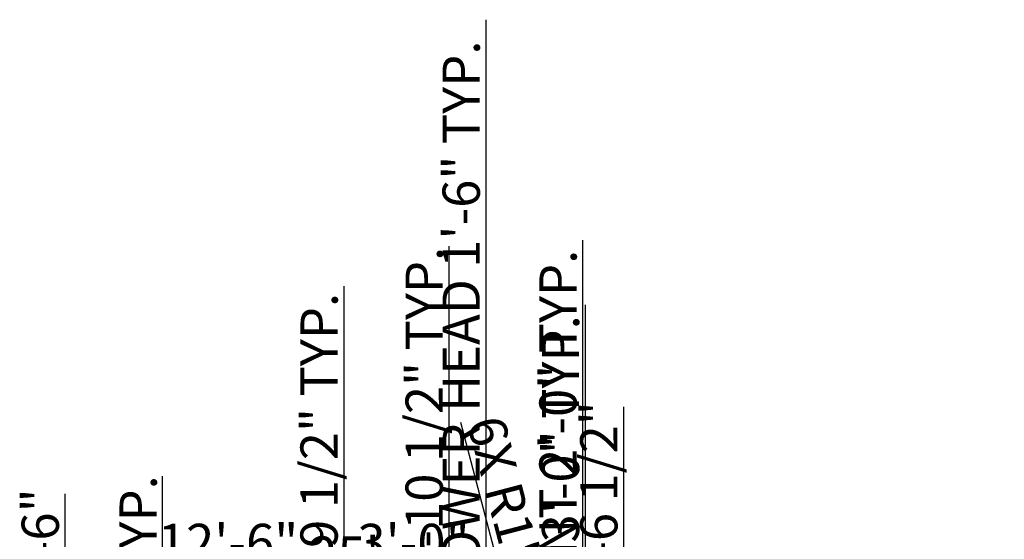
# Model space of a CAD drawing. Units: inches. Extents: x 830 to 1639, y 2591 to 3595.
# Tile 7 of 7: x 922 to 1557, y 3260 to 3595. Entities that reach past the tile are written whole.
import ezdxf

# ---------------------------------------------------------------- set-up
doc = ezdxf.new("R2010")
doc.units = ezdxf.units.IN
doc.layers.add('A-ANNO-DIMS', color=2, linetype='Continuous', lineweight=18)
doc.styles.get("Standard").update_dxf_attribs({"font": 'arial.ttf'})
doc.dimstyles.new('ISO-25', dxfattribs={"dimtxt": 24, "dimasz": 12, "dimexe": 1.25, "dimexo": 0.625, "dimtad": 1, "dimdec": 0, "dimlunit": 3, "dimtxsty": 'Standard', "dimcen": 2.5, "dimadec": 0, "dimazin": 0, "dimtfac": 1, "dimtdec": 0, "dimtmove": 0, "dimatfit": 3, "dimfxl": 1, "dimarcsym": 0})

# ---------------------------------------------------------------- blocks, each defined once
blk = doc.blocks.new('*D15')
at = {"layer": 'A-ANNO-DIMS', "color": 0, "lineweight": -2, "transparency": 16777216}
for p, q in [((981.59, 3212.71), (981.59, 3235.25)), ((993.59, 3234), (1269.59, 3234)), ((1281.59, 3212.71), (1281.59, 3235.25))]:
    blk.add_line(p, q, dxfattribs=at)
at = {"layer": 'A-ANNO-DIMS', "color": 0, "transparency": 16777216}
for points in [[(993.59, 3236), (993.59, 3232), (981.59, 3234)], [(1269.59, 3236), (1269.59, 3232), (1281.59, 3234)]]:
    blk.add_solid(points, dxfattribs=at)
at = {"layer": 'Defpoints', "color": 0, "transparency": 16777216}
for p in [(1281.59, 3234), (981.59, 3212.09), (1281.59, 3212.09)]:
    blk.add_point(p, dxfattribs=at)
at = {"layer": 'A-ANNO-DIMS', "color": 0, "transparency": 16777216, "insert": (1131.59, 3246.88), "char_height": 24, "attachment_point": 5}
blk.add_mtext("25'", dxfattribs=at)
blk = doc.blocks.new('*D22')
at = {"layer": 'A-ANNO-DIMS', "color": 0, "lineweight": -2, "transparency": 16777216}
for p, q in [((1286.99, 3094.42), (1286.99, 3411.37)), ((1282.21, 3094.42), (1288.24, 3094.42)), ((1286.99, 3070.42), (1286.99, 3082.42)), ((1282.21, 3058.42), (1288.24, 3058.42))]:
    blk.add_line(p, q, dxfattribs=at)
at = {"layer": 'A-ANNO-DIMS', "color": 0, "transparency": 16777216}
for points in [[(1284.99, 3082.42), (1288.99, 3082.42), (1286.99, 3094.42)], [(1284.99, 3070.42), (1288.99, 3070.42), (1286.99, 3058.42)]]:
    blk.add_solid(points, dxfattribs=at)
at = {"layer": 'Defpoints', "color": 0, "transparency": 16777216}
for p in [(1281.59, 3094.42), (1286.99, 3094.42), (1281.59, 3058.42)]:
    blk.add_point(p, dxfattribs=at)
at = {"layer": 'A-ANNO-DIMS', "color": 0, "transparency": 16777216, "insert": (1273.94, 3258.89), "char_height": 24, "attachment_point": 5, "rotation": 90}
blk.add_mtext('WINDOW 3\'-0" TYP.', dxfattribs=at)
blk = doc.blocks.new('*D24')
at = {"layer": 'A-ANNO-DIMS', "color": 0, "lineweight": -2, "transparency": 16777216}
for p, q in [((1285.19, 3193.45), (1285.19, 3452.97)), ((1282.21, 3181.45), (1286.44, 3181.45)), ((1285.19, 3157.45), (1285.19, 3181.45)), ((1282.21, 3157.45), (1286.44, 3157.45)), ((1285.19, 3145.45), (1285.19, 3133.45))]:
    blk.add_line(p, q, dxfattribs=at)
at = {"layer": 'A-ANNO-DIMS', "color": 0, "transparency": 16777216}
for points in [[(1283.19, 3193.45), (1287.19, 3193.45), (1285.19, 3181.45)], [(1283.19, 3145.45), (1287.19, 3145.45), (1285.19, 3157.45)]]:
    blk.add_solid(points, dxfattribs=at)
at = {"layer": 'Defpoints', "color": 0, "transparency": 16777216}
for p in [(1281.59, 3181.45), (1285.19, 3181.45), (1281.59, 3157.45)]:
    blk.add_point(p, dxfattribs=at)
at = {"layer": 'A-ANNO-DIMS', "color": 0, "transparency": 16777216, "insert": (1272.31, 3329.21), "char_height": 24, "attachment_point": 5, "rotation": 90}
blk.add_mtext('VENT 2\'-0" TYP.', dxfattribs=at)
blk = doc.blocks.new('*D27')
at = {"layer": 'A-ANNO-DIMS', "color": 0, "lineweight": -2, "transparency": 16777216}
for p, q in [((1014.41, 3143.5), (1014.41, 3300.79)), ((1011.93, 3131.5), (1015.66, 3131.5)), ((1014.41, 3112.26), (1014.41, 3131.5)), ((1011.93, 3112.26), (1015.66, 3112.26)), ((1014.41, 3100.26), (1014.41, 3088.26))]:
    blk.add_line(p, q, dxfattribs=at)
at = {"layer": 'A-ANNO-DIMS', "color": 0, "transparency": 16777216}
for points in [[(1012.41, 3143.5), (1016.41, 3143.5), (1014.41, 3131.5)], [(1012.41, 3100.26), (1016.41, 3100.26), (1014.41, 3112.26)]]:
    blk.add_solid(points, dxfattribs=at)
at = {"layer": 'Defpoints', "color": 0, "transparency": 16777216}
for p in [(1011.31, 3131.5), (1014.41, 3131.5), (1011.31, 3112.26)]:
    blk.add_point(p, dxfattribs=at)
at = {"layer": 'A-ANNO-DIMS', "color": 0, "transparency": 16777216, "insert": (1001.73, 3228.15), "char_height": 24, "attachment_point": 5, "rotation": 90}
blk.add_mtext('1\'-7" TYP.', dxfattribs=at)
blk = doc.blocks.new('*D34')
at = {"layer": 'A-ANNO-DIMS', "color": 0, "lineweight": -2, "transparency": 16777216}
for p, q in [((1189.9, 3205.85), (1177.9, 3205.85)), ((1201.9, 3203.69), (1201.9, 3207.1)), ((1201.9, 3205.85), (1220.46, 3205.85)), ((1220.46, 3203.69), (1220.46, 3207.1)), ((1232.46, 3205.85), (1556.8, 3205.85))]:
    blk.add_line(p, q, dxfattribs=at)
at = {"layer": 'A-ANNO-DIMS', "color": 0, "transparency": 16777216}
for points in [[(1189.9, 3207.85), (1189.9, 3203.85), (1201.9, 3205.85)], [(1232.46, 3207.85), (1232.46, 3203.85), (1220.46, 3205.85)]]:
    blk.add_solid(points, dxfattribs=at)
at = {"layer": 'Defpoints', "color": 0, "transparency": 16777216}
for p in [(1220.46, 3205.85), (1201.9, 3203.07), (1220.46, 3203.07)]:
    blk.add_point(p, dxfattribs=at)
at = {"layer": 'A-ANNO-DIMS', "color": 0, "transparency": 16777216, "insert": (1400.63, 3218.88), "char_height": 24, "attachment_point": 5}
blk.add_mtext('BASIN 1\'-6 1/2" TYP.', dxfattribs=at)
blk = doc.blocks.new('*D35')
at = {"layer": 'A-ANNO-DIMS', "color": 0, "lineweight": -2, "transparency": 16777216}
for p, q in [((1199.11, 3215.07), (1199.11, 3449.18)), ((1201.27, 3203.07), (1197.86, 3203.07)), ((1199.11, 3192.62), (1199.11, 3203.07)), ((1201.27, 3192.62), (1197.86, 3192.62)), ((1199.11, 3180.62), (1199.11, 3168.62))]:
    blk.add_line(p, q, dxfattribs=at)
at = {"layer": 'A-ANNO-DIMS', "color": 0, "transparency": 16777216}
for points in [[(1197.11, 3215.07), (1201.11, 3215.07), (1199.11, 3203.07)], [(1197.11, 3180.62), (1201.11, 3180.62), (1199.11, 3192.62)]]:
    blk.add_solid(points, dxfattribs=at)
at = {"layer": 'Defpoints', "color": 0, "transparency": 16777216}
for p in [(1199.11, 3203.07), (1201.9, 3203.07), (1201.9, 3192.62)]:
    blk.add_point(p, dxfattribs=at)
at = {"layer": 'A-ANNO-DIMS', "color": 0, "transparency": 16777216, "insert": (1186.08, 3338.12), "char_height": 24, "attachment_point": 5, "rotation": 90}
blk.add_mtext('0\'-10 1/2" TYP.', dxfattribs=at)
blk = doc.blocks.new('*D38')
at = {"layer": 'A-ANNO-DIMS', "color": 0, "lineweight": -2, "transparency": 16777216}
for p, q in [((1222.96, 3173.04), (1222.96, 3595.13)), ((1220.89, 3161.04), (1224.21, 3161.04)), ((1222.96, 3143.09), (1222.96, 3161.04)), ((1220.89, 3143.09), (1224.21, 3143.09)), ((1222.96, 3131.09), (1222.96, 3119.09))]:
    blk.add_line(p, q, dxfattribs=at)
at = {"layer": 'A-ANNO-DIMS', "color": 0, "transparency": 16777216}
for points in [[(1220.96, 3173.04), (1224.96, 3173.04), (1222.96, 3161.04)], [(1220.96, 3131.09), (1224.96, 3131.09), (1222.96, 3143.09)]]:
    blk.add_solid(points, dxfattribs=at)
at = {"layer": 'Defpoints', "color": 0, "transparency": 16777216}
for p in [(1220.27, 3161.04), (1222.96, 3161.04), (1220.27, 3143.09)]:
    blk.add_point(p, dxfattribs=at)
at = {"layer": 'A-ANNO-DIMS', "color": 0, "transparency": 16777216, "insert": (1209.92, 3390.09), "char_height": 24, "attachment_point": 5, "rotation": 90}
blk.add_mtext('SHOWER HEAD 1\'-6" TYP.', dxfattribs=at)
blk = doc.blocks.new('*D40')
at = {"layer": 'A-ANNO-DIMS', "color": 0, "lineweight": -2, "transparency": 16777216}
for p, q in [((1131.38, 3125.32), (1131.38, 3423.36)), ((1116.15, 3125.32), (1132.63, 3125.32)), ((1131.38, 3031.63), (1131.38, 3113.32)), ((1116.15, 3019.63), (1132.63, 3019.63))]:
    blk.add_line(p, q, dxfattribs=at)
at = {"layer": 'A-ANNO-DIMS', "color": 0, "transparency": 16777216}
for points in [[(1129.38, 3113.32), (1133.38, 3113.32), (1131.38, 3125.32)], [(1129.38, 3031.63), (1133.38, 3031.63), (1131.38, 3019.63)]]:
    blk.add_solid(points, dxfattribs=at)
at = {"layer": 'Defpoints', "color": 0, "transparency": 16777216}
for p in [(1115.52, 3125.32), (1131.38, 3125.32), (1115.52, 3019.63)]:
    blk.add_point(p, dxfattribs=at)
at = {"layer": 'A-ANNO-DIMS', "color": 0, "transparency": 16777216, "insert": (1118.34, 3280.34), "char_height": 24, "attachment_point": 5, "rotation": 90}
blk.add_mtext('RUG 8\'-9 1/2" TYP.', dxfattribs=at)
blk = doc.blocks.new('*D49')
at = {"layer": 'A-ANNO-DIMS', "color": 0, "lineweight": -2, "transparency": 16777216}
for p, q in [((1095.59, 2991.71), (1095.59, 3243.39)), ((1131.59, 2992.51), (1131.59, 3243.39)), ((1107.59, 3242.14), (1119.59, 3242.14)), ((1131.59, 3242.14), (1208.62, 3242.14))]:
    blk.add_line(p, q, dxfattribs=at)
at = {"layer": 'A-ANNO-DIMS', "color": 0, "transparency": 16777216}
for points in [[(1107.59, 3244.14), (1107.59, 3240.14), (1095.59, 3242.14)], [(1119.59, 3244.14), (1119.59, 3240.14), (1131.59, 3242.14)]]:
    blk.add_solid(points, dxfattribs=at)
at = {"layer": 'Defpoints', "color": 0, "transparency": 16777216}
for p in [(1131.59, 3242.14), (1095.59, 2991.09), (1131.59, 2991.89)]:
    blk.add_point(p, dxfattribs=at)
at = {"layer": 'A-ANNO-DIMS', "color": 0, "transparency": 16777216, "insert": (1176.11, 3255.02), "char_height": 24, "attachment_point": 5}
blk.add_mtext('3\'-0"', dxfattribs=at)
blk = doc.blocks.new('*D58')
at = {"layer": 'A-ANNO-DIMS', "color": 0, "lineweight": -2, "transparency": 16777216}
for p, q in [((981.59, 3212.71), (981.59, 3243.39)), ((1131.59, 3203.71), (1131.59, 3243.39)), ((993.59, 3242.14), (1119.59, 3242.14))]:
    blk.add_line(p, q, dxfattribs=at)
at = {"layer": 'A-ANNO-DIMS', "color": 0, "transparency": 16777216}
for points in [[(993.59, 3244.14), (993.59, 3240.14), (981.59, 3242.14)], [(1119.59, 3244.14), (1119.59, 3240.14), (1131.59, 3242.14)]]:
    blk.add_solid(points, dxfattribs=at)
at = {"layer": 'Defpoints', "color": 0, "transparency": 16777216}
for p in [(1131.59, 3242.14), (981.59, 3212.09), (1131.59, 3203.09)]:
    blk.add_point(p, dxfattribs=at)
at = {"layer": 'A-ANNO-DIMS', "color": 0, "transparency": 16777216, "insert": (1056.59, 3255.02), "char_height": 24, "attachment_point": 5}
blk.add_mtext('12\'-6"', dxfattribs=at)
blk = doc.blocks.new('*D69')
at = {"layer": 'A-ANNO-DIMS', "color": 0, "lineweight": -2, "transparency": 16777216}
for p, q in [((951.54, 3212.09), (951.54, 3289.54)), ((980.96, 3212.09), (950.29, 3212.09)), ((951.54, 3194.32), (951.54, 3200.09)), ((980.96, 3182.32), (950.29, 3182.32))]:
    blk.add_line(p, q, dxfattribs=at)
at = {"layer": 'A-ANNO-DIMS', "color": 0, "transparency": 16777216}
for points in [[(949.54, 3200.09), (953.54, 3200.09), (951.54, 3212.09)], [(949.54, 3194.32), (953.54, 3194.32), (951.54, 3182.32)]]:
    blk.add_solid(points, dxfattribs=at)
at = {"layer": 'Defpoints', "color": 0, "transparency": 16777216}
for p in [(951.54, 3212.09), (981.59, 3212.09), (981.59, 3182.32)]:
    blk.add_point(p, dxfattribs=at)
at = {"layer": 'A-ANNO-DIMS', "color": 0, "transparency": 16777216, "insert": (938.66, 3256.82), "char_height": 24, "attachment_point": 5, "rotation": 90}
blk.add_mtext('2\'-6"', dxfattribs=at)
blk = doc.blocks.new('*D70')
at = {"layer": 'A-ANNO-DIMS', "color": 0, "lineweight": -2, "transparency": 16777216}
for p, q in [((1311.64, 3212.09), (1311.64, 3345.47)), ((1282.21, 3212.09), (1312.89, 3212.09)), ((1311.64, 3193.45), (1311.64, 3200.09)), ((1282.21, 3181.45), (1312.89, 3181.45))]:
    blk.add_line(p, q, dxfattribs=at)
at = {"layer": 'A-ANNO-DIMS', "color": 0, "transparency": 16777216}
for points in [[(1309.64, 3200.09), (1313.64, 3200.09), (1311.64, 3212.09)], [(1309.64, 3193.45), (1313.64, 3193.45), (1311.64, 3181.45)]]:
    blk.add_solid(points, dxfattribs=at)
at = {"layer": 'Defpoints', "color": 0, "transparency": 16777216}
for p in [(1281.59, 3212.09), (1311.64, 3212.09), (1281.59, 3181.45)]:
    blk.add_point(p, dxfattribs=at)
at = {"layer": 'A-ANNO-DIMS', "color": 0, "transparency": 16777216, "insert": (1298.61, 3284.78), "char_height": 24, "attachment_point": 5, "rotation": 90}
blk.add_mtext('2\'-6 1/2"', dxfattribs=at)
blk = doc.blocks.new('*D75')
at = {"layer": 'A-ANNO-DIMS', "color": 0, "lineweight": -2, "transparency": 16777216}
for p, q in [((1206.32, 3335.67), (1244.87, 3188.93)), ((1251.01, 3165.56), (1247.92, 3177.33))]:
    blk.add_line(p, q, dxfattribs=at)
at = {"layer": 'A-ANNO-DIMS', "color": 0, "transparency": 16777216}
blk.add_solid([(1246.8, 3189.44), (1242.93, 3188.43), (1247.92, 3177.33)], dxfattribs=at)
at = {"layer": 'Defpoints', "color": 0, "transparency": 16777216}
for p in [(1247.92, 3177.33), (1251.01, 3165.56)]:
    blk.add_point(p, dxfattribs=at)
at = {"layer": 'A-ANNO-DIMS', "color": 0, "transparency": 16777216, "insert": (1236.52, 3271.38), "char_height": 24, "attachment_point": 5, "rotation": 284.72029}
blk.add_mtext('6X R1\'-0"', dxfattribs=at)

msp = doc.modelspace()

# ---------------------------------------------------------------- dimensions: what is measured, and where the dimension line sits
at = {"layer": 'A-ANNO-DIMS'}
for base, p1, p2, text, picture, middle in [((1222.9595, 3161.0435), (1220.2661, 3143.0874), (1220.2661, 3161.0435), 'SHOWER HEAD <> TYP.', '*D38', (1209.917, 3390.086)), ((1285.19, 3181.45), (1281.59, 3157.45), (1281.59, 3181.45), 'VENT <> TYP.', '*D24', (1272.31, 3329.21)), ((1199.1117, 3203.0656), (1201.8966, 3192.6174), (1201.8966, 3203.0656), '<> TYP.', '*D35', (1186.0775, 3338.1217)), ((1131.38, 3125.32), (1115.52, 3019.63), (1115.52, 3125.32), 'RUG <> TYP.', '*D40', (1118.34, 3280.34)), ((1286.99, 3094.42), (1281.59, 3058.42), (1281.59, 3094.42), 'WINDOW <> TYP.', '*D22', (1273.94, 3258.89)), ((1014.41, 3131.5), (1011.31, 3112.26), (1011.31, 3131.5), '<> TYP.', '*D27', (1001.73, 3228.15))]:
    dim = msp.add_linear_dim(base=base, p1=p1, p2=p2, angle=90, text=text, dimstyle='ISO-25', override={"dimdec": 1, "dimlfac": 1, "dimrnd": 0, "dimzin": 1, "dimdsep": 46, "dimlunit": 4, "dimfrac": 2}, dxfattribs=at)
    dim.commit()
    dim.dimension.update_dxf_attribs({"geometry": picture, "text_midpoint": middle})
for base, p1, p2, picture, middle in [((1311.64, 3212.09), (1281.59, 3181.45), (1281.59, 3212.09), '*D70', (1298.61, 3284.78)), ((951.54, 3212.09), (981.59, 3182.32), (981.59, 3212.09), '*D69', (938.66, 3256.82))]:
    dim = msp.add_linear_dim(base=base, p1=p1, p2=p2, angle=90, dimstyle='ISO-25', override={"dimdec": 1, "dimlfac": 1, "dimrnd": 0, "dimzin": 1, "dimdsep": 46, "dimlunit": 4, "dimfrac": 2}, dxfattribs=at)
    dim.commit()
    dim.dimension.update_dxf_attribs({"geometry": picture, "text_midpoint": middle})
dim = msp.add_radius_dim(center=(1251.01, 3165.56), mpoint=(1247.92, 3177.33), text='6X <>', dimstyle='ISO-25', override={"dimdec": 1, "dimlfac": 1, "dimrnd": 0, "dimzin": 1, "dimdsep": 46, "dimlunit": 4, "dimfrac": 2}, dxfattribs=at)
dim.commit()
dim.dimension.update_dxf_attribs({"geometry": '*D75', "text_midpoint": (1236.52, 3271.38)})
dim = msp.add_linear_dim(base=(1220.46, 3205.85), p1=(1201.9, 3203.07), p2=(1220.46, 3203.07), text='BASIN <> TYP.', dimstyle='ISO-25', override={"dimdec": 1, "dimlfac": 1, "dimrnd": 0, "dimzin": 1, "dimdsep": 46, "dimlunit": 4, "dimfrac": 2}, dxfattribs=at)
dim.commit()
dim.dimension.update_dxf_attribs({"geometry": '*D34', "text_midpoint": (1400.63, 3218.88)})
for base, p1, p2, override, picture, middle in [((1131.59, 3242.14), (981.59, 3212.09), (1131.59, 3203.09), {"dimdec": 1, "dimlfac": 1, "dimrnd": 0, "dimzin": 1, "dimdsep": 46, "dimlunit": 4, "dimfrac": 2}, '*D58', (1056.59, 3255.02)), ((1131.59, 3242.14), (1095.59, 2991.09), (1131.59, 2991.89), {"dimdec": 1, "dimlfac": 1, "dimrnd": 0, "dimzin": 1, "dimdsep": 46, "dimlunit": 4, "dimfrac": 2}, '*D49', (1176.11, 3255.02)), ((1281.59, 3234), (981.59, 3212.09), (1281.59, 3212.09), {"dimclrd": 0, "dimclre": 0, "dimclrt": 0}, '*D15', (1131.59, 3246.88))]:
    dim = msp.add_linear_dim(base=base, p1=p1, p2=p2, dimstyle='ISO-25', override=override, dxfattribs=at)
    dim.commit()
    dim.dimension.update_dxf_attribs({"geometry": picture, "text_midpoint": middle})

doc.saveas('drawing.dxf')
